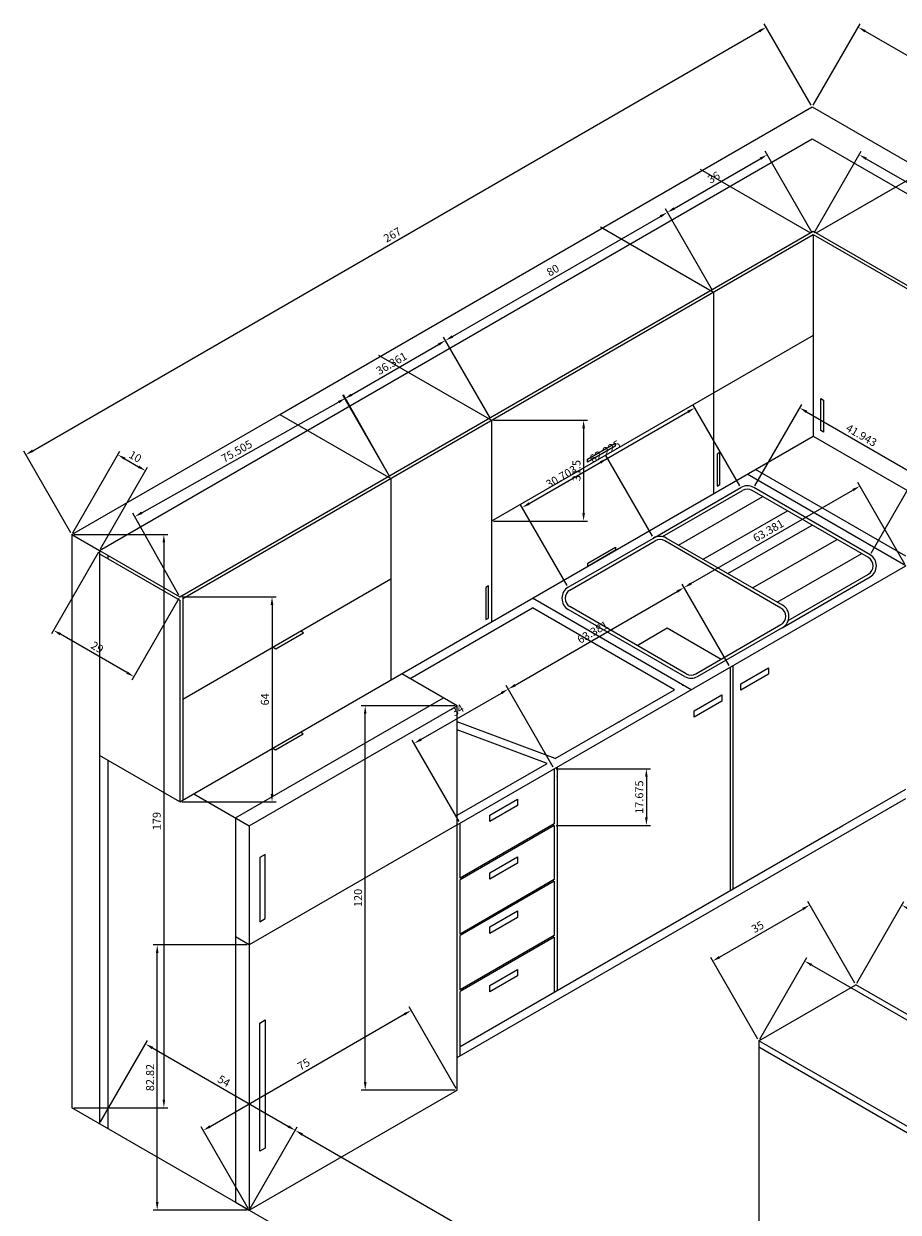
# Model space of a CAD drawing. Units: centimetres. Extents: x 239489 to 240034, y 95136 to 95693.
# Tile 2 of 4: x 239489 to 239762, y 95322 to 95693. Entities that reach past the tile are written whole.
import ezdxf

# ---------------------------------------------------------------- set-up
doc = ezdxf.new("R2010")
doc.units = ezdxf.units.CM
doc.layers.add('A-ANNO-DIMS', color=2, linetype='Continuous', lineweight=18)
doc.layers.add('A-FLOR-CASE', color=7, linetype='Continuous', lineweight=25)
doc.styles.get("Standard").update_dxf_attribs({"font": 'arial.ttf'})
doc.dimstyles.new('ISO-25', dxfattribs={"dimtxt": 2.5, "dimasz": 2.5, "dimexe": 1.25, "dimexo": 0.625, "dimtad": 1, "dimdec": 1, "dimdsep": 46, "dimtxsty": 'Standard', "dimcen": 2.5, "dimadec": 0, "dimazin": 0, "dimtfac": 1, "dimtdec": 1, "dimtmove": 0, "dimatfit": 3, "dimfxl": 1, "dimarcsym": 0})

# ---------------------------------------------------------------- blocks, each defined once
blk = doc.blocks.new('HANDLE-DOOR')
for p, q in [((0.87, 10.5), (0, 10)), ((0, 10), (0, 0)), ((0.87, 0.5), (0.87, 10.5)), ((0, 0), (0.87, 0.5))]:
    blk.add_line(p, q)
blk = doc.blocks.new('HANDLE-DRAWER')
for p, q in [((0, 2), (8.66, 7)), ((8.66, 5), (0, 0)), ((8.66, 7), (8.66, 5)), ((0, 0), (0, 2))]:
    blk.add_line(p, q)
blk = doc.blocks.new('*D4')
at = {"layer": 'A-ANNO-DIMS', "color": 0, "lineweight": -2, "transparency": 16777216}
for p, q in [((239734.94, 95667.89), (239720.25, 95693.33)), ((239491.82, 95560), (239718.71, 95691)), ((239503.71, 95534.39), (239489.03, 95559.83))]:
    blk.add_line(p, q, dxfattribs=at)
at = {"layer": 'A-ANNO-DIMS', "color": 0, "transparency": 16777216}
for points in [[(239718.51, 95691.36), (239718.92, 95690.64), (239720.88, 95692.25)], [(239491.61, 95560.36), (239492.02, 95559.64), (239489.65, 95558.75)]]:
    blk.add_solid(points, dxfattribs=at)
at = {"layer": 'Defpoints', "color": 0, "transparency": 16777216}
for p in [(239720.88, 95692.25), (239735.25, 95667.35), (239504.03, 95533.85)]:
    blk.add_point(p, dxfattribs=at)
at = {"layer": 'A-ANNO-DIMS', "color": 0, "transparency": 16777216, "insert": (239604.31, 95627.15), "char_height": 2.5, "attachment_point": 5, "rotation": 30}
blk.add_mtext('267', dxfattribs=at)
blk = doc.blocks.new('*D5')
at = {"layer": 'A-ANNO-DIMS', "color": 0, "lineweight": -2, "transparency": 16777216}
for p, q in [((239735.57, 95667.89), (239750.25, 95693.33)), ((239751.79, 95691), (239980.86, 95558.75)), ((239968.97, 95533.14), (239983.65, 95558.58))]:
    blk.add_line(p, q, dxfattribs=at)
at = {"layer": 'A-ANNO-DIMS', "color": 0, "transparency": 16777216}
for points in [[(239752, 95691.36), (239751.59, 95690.64), (239749.63, 95692.25)], [(239981.07, 95559.11), (239980.65, 95558.39), (239983.03, 95557.5)]]:
    blk.add_solid(points, dxfattribs=at)
at = {"layer": 'Defpoints', "color": 0, "transparency": 16777216}
for p in [(239735.25, 95667.35), (239983.03, 95557.5), (239968.65, 95532.6)]:
    blk.add_point(p, dxfattribs=at)
at = {"layer": 'A-ANNO-DIMS', "color": 0, "transparency": 16777216, "insert": (239867.28, 95626.52), "char_height": 2.5, "attachment_point": 5, "rotation": 330}
blk.add_mtext('269.505', dxfattribs=at)
blk = doc.blocks.new('*D7')
at = {"layer": 'A-ANNO-DIMS', "color": 0, "lineweight": -2, "transparency": 16777216}
for p, q in [((239504.65, 95533.85), (239534.03, 95533.85)), ((239532.78, 95531.35), (239532.78, 95357.35)), ((239504.65, 95354.85), (239534.03, 95354.85))]:
    blk.add_line(p, q, dxfattribs=at)
at = {"layer": 'A-ANNO-DIMS', "color": 0, "transparency": 16777216}
for points in [[(239532.36, 95531.35), (239533.19, 95531.35), (239532.78, 95533.85)], [(239532.36, 95357.35), (239533.19, 95357.35), (239532.78, 95354.85)]]:
    blk.add_solid(points, dxfattribs=at)
at = {"layer": 'Defpoints', "color": 0, "transparency": 16777216}
for p in [(239504.03, 95533.85), (239504.03, 95354.85), (239532.78, 95354.85)]:
    blk.add_point(p, dxfattribs=at)
at = {"layer": 'A-ANNO-DIMS', "color": 0, "transparency": 16777216, "insert": (239530.87, 95444.35), "char_height": 2.5, "attachment_point": 5, "rotation": 90}
blk.add_mtext('179', dxfattribs=at)
blk = doc.blocks.new('*D8')
at = {"layer": 'A-ANNO-DIMS', "color": 0, "lineweight": -2, "transparency": 16777216}
for p, q in [((239504.34, 95534.39), (239519.03, 95559.83)), ((239513, 95529.39), (239527.69, 95554.83)), ((239520.57, 95557.5), (239524.9, 95555))]:
    blk.add_line(p, q, dxfattribs=at)
at = {"layer": 'A-ANNO-DIMS', "color": 0, "transparency": 16777216}
for points in [[(239520.77, 95557.86), (239520.36, 95557.14), (239518.4, 95558.75)], [(239525.1, 95555.36), (239524.69, 95554.64), (239527.06, 95553.75)]]:
    blk.add_solid(points, dxfattribs=at)
at = {"layer": 'Defpoints', "color": 0, "transparency": 16777216}
for p in [(239527.06, 95553.75), (239504.03, 95533.85), (239512.69, 95528.85)]:
    blk.add_point(p, dxfattribs=at)
at = {"layer": 'A-ANNO-DIMS', "color": 0, "transparency": 16777216, "insert": (239523.68, 95557.9), "char_height": 2.5, "attachment_point": 5, "rotation": 330}
blk.add_mtext('10', dxfattribs=at)
blk = doc.blocks.new('*D10')
at = {"layer": 'A-ANNO-DIMS', "color": 0, "lineweight": -2, "transparency": 16777216}
for p, q in [((239513, 95350.39), (239527.69, 95375.83)), ((239529.23, 95373.5), (239571.66, 95349)), ((239559.76, 95323.39), (239574.45, 95348.83))]:
    blk.add_line(p, q, dxfattribs=at)
at = {"layer": 'A-ANNO-DIMS', "color": 0, "transparency": 16777216}
for points in [[(239529.43, 95373.86), (239529.02, 95373.14), (239527.06, 95374.75)], [(239571.87, 95349.36), (239571.45, 95348.64), (239573.83, 95347.75)]]:
    blk.add_solid(points, dxfattribs=at)
at = {"layer": 'Defpoints', "color": 0, "transparency": 16777216}
for p in [(239512.69, 95349.85), (239573.83, 95347.75), (239559.45, 95322.85)]:
    blk.add_point(p, dxfattribs=at)
at = {"layer": 'A-ANNO-DIMS', "color": 0, "transparency": 16777216, "insert": (239551.39, 95362.89), "char_height": 2.5, "attachment_point": 5, "rotation": 330}
blk.add_mtext('54', dxfattribs=at)
blk = doc.blocks.new('*D11')
at = {"layer": 'A-ANNO-DIMS', "color": 0, "lineweight": -2, "transparency": 16777216}
for p, q in [((239559.76, 95323.39), (239574.45, 95348.83)), ((239575.99, 95346.5), (239730.75, 95257.15)), ((239718.86, 95231.54), (239733.54, 95256.98))]:
    blk.add_line(p, q, dxfattribs=at)
at = {"layer": 'A-ANNO-DIMS', "color": 0, "transparency": 16777216}
for points in [[(239576.2, 95346.86), (239575.78, 95346.14), (239573.83, 95347.75)], [(239730.96, 95257.51), (239730.55, 95256.79), (239732.92, 95255.9)]]:
    blk.add_solid(points, dxfattribs=at)
at = {"layer": 'Defpoints', "color": 0, "transparency": 16777216}
for p in [(239559.45, 95322.85), (239732.92, 95255.9), (239718.54, 95231)]:
    blk.add_point(p, dxfattribs=at)
at = {"layer": 'A-ANNO-DIMS', "color": 0, "transparency": 16777216, "insert": (239654.32, 95303.47), "char_height": 2.5, "attachment_point": 5, "rotation": 330}
blk.add_mtext('183.705', dxfattribs=at)
blk = doc.blocks.new('*D12')
at = {"layer": 'A-ANNO-DIMS', "color": 0, "lineweight": -2, "transparency": 16777216}
for p, q in [((239624.09, 95360.89), (239609.4, 95386.33)), ((239547.24, 95349), (239607.86, 95384)), ((239559.14, 95323.39), (239544.45, 95348.83))]:
    blk.add_line(p, q, dxfattribs=at)
at = {"layer": 'A-ANNO-DIMS', "color": 0, "transparency": 16777216}
for points in [[(239607.66, 95384.36), (239608.07, 95383.64), (239610.03, 95385.25)], [(239547.03, 95349.36), (239547.45, 95348.64), (239545.08, 95347.75)]]:
    blk.add_solid(points, dxfattribs=at)
at = {"layer": 'Defpoints', "color": 0, "transparency": 16777216}
for p in [(239610.03, 95385.25), (239624.4, 95360.35), (239559.45, 95322.85)]:
    blk.add_point(p, dxfattribs=at)
at = {"layer": 'A-ANNO-DIMS', "color": 0, "transparency": 16777216, "insert": (239576.6, 95368.14), "char_height": 2.5, "attachment_point": 5, "rotation": 30}
blk.add_mtext('75', dxfattribs=at)
blk = doc.blocks.new('*D13')
at = {"layer": 'A-ANNO-DIMS', "color": 0, "lineweight": -2, "transparency": 16777216}
for p, q in [((239623.78, 95480.35), (239594.4, 95480.35)), ((239595.65, 95362.85), (239595.65, 95477.85)), ((239623.78, 95360.35), (239594.4, 95360.35))]:
    blk.add_line(p, q, dxfattribs=at)
at = {"layer": 'A-ANNO-DIMS', "color": 0, "transparency": 16777216}
for points in [[(239595.24, 95477.85), (239596.07, 95477.85), (239595.65, 95480.35)], [(239595.24, 95362.85), (239596.07, 95362.85), (239595.65, 95360.35)]]:
    blk.add_solid(points, dxfattribs=at)
at = {"layer": 'Defpoints', "color": 0, "transparency": 16777216}
for p in [(239595.65, 95480.35), (239624.4, 95480.35), (239624.4, 95360.35)]:
    blk.add_point(p, dxfattribs=at)
at = {"layer": 'A-ANNO-DIMS', "color": 0, "transparency": 16777216, "insert": (239593.75, 95420.35), "char_height": 2.5, "attachment_point": 5, "rotation": 90}
blk.add_mtext('120', dxfattribs=at)
blk = doc.blocks.new('*D14')
at = {"layer": 'A-ANNO-DIMS', "color": 0, "lineweight": -2, "transparency": 16777216}
for p, q in [((239558.83, 95405.67), (239529.45, 95405.67)), ((239530.7, 95325.35), (239530.7, 95403.17)), ((239558.83, 95322.85), (239529.45, 95322.85))]:
    blk.add_line(p, q, dxfattribs=at)
at = {"layer": 'A-ANNO-DIMS', "color": 0, "transparency": 16777216}
for points in [[(239530.28, 95403.17), (239531.12, 95403.17), (239530.7, 95405.67)], [(239530.28, 95325.35), (239531.12, 95325.35), (239530.7, 95322.85)]]:
    blk.add_solid(points, dxfattribs=at)
at = {"layer": 'Defpoints', "color": 0, "transparency": 16777216}
for p in [(239530.7, 95405.67), (239559.45, 95405.67), (239559.45, 95322.85)]:
    blk.add_point(p, dxfattribs=at)
at = {"layer": 'A-ANNO-DIMS', "color": 0, "transparency": 16777216, "insert": (239528.8, 95364.26), "char_height": 2.5, "attachment_point": 5, "rotation": 90}
blk.add_mtext('82.82', dxfattribs=at)
blk = doc.blocks.new('*D15')
at = {"layer": 'A-ANNO-DIMS', "color": 0, "lineweight": -2, "transparency": 16777216}
for p, q in [((239538.43, 95514.35), (239567.8, 95514.35)), ((239566.55, 95511.85), (239566.55, 95452.85)), ((239538.43, 95450.35), (239567.8, 95450.35))]:
    blk.add_line(p, q, dxfattribs=at)
at = {"layer": 'A-ANNO-DIMS', "color": 0, "transparency": 16777216}
for points in [[(239566.13, 95511.85), (239566.97, 95511.85), (239566.55, 95514.35)], [(239566.13, 95452.85), (239566.97, 95452.85), (239566.55, 95450.35)]]:
    blk.add_solid(points, dxfattribs=at)
at = {"layer": 'Defpoints', "color": 0, "transparency": 16777216}
for p in [(239537.8, 95514.35), (239537.8, 95450.35), (239566.55, 95450.35)]:
    blk.add_point(p, dxfattribs=at)
at = {"layer": 'A-ANNO-DIMS', "color": 0, "transparency": 16777216, "insert": (239564.65, 95482.35), "char_height": 2.5, "attachment_point": 5, "rotation": 90}
blk.add_mtext('64', dxfattribs=at)
blk = doc.blocks.new('*D16')
at = {"layer": 'A-ANNO-DIMS', "color": 0, "lineweight": -2, "transparency": 16777216}
for p, q in [((239512.37, 95528.31), (239497.69, 95502.87)), ((239537.49, 95513.81), (239522.8, 95488.37)), ((239521.26, 95490.7), (239500.48, 95502.7))]:
    blk.add_line(p, q, dxfattribs=at)
at = {"layer": 'A-ANNO-DIMS', "color": 0, "transparency": 16777216}
for points in [[(239500.68, 95503.06), (239500.27, 95502.34), (239498.31, 95503.95)], [(239521.47, 95491.06), (239521.05, 95490.34), (239523.43, 95489.45)]]:
    blk.add_solid(points, dxfattribs=at)
at = {"layer": 'Defpoints', "color": 0, "transparency": 16777216}
for p in [(239512.69, 95528.85), (239537.8, 95514.35), (239498.31, 95503.95)]:
    blk.add_point(p, dxfattribs=at)
at = {"layer": 'A-ANNO-DIMS', "color": 0, "transparency": 16777216, "insert": (239511.82, 95498.35), "char_height": 2.5, "attachment_point": 5, "rotation": 330}
blk.add_mtext('29', dxfattribs=at)
blk = doc.blocks.new('*D17')
at = {"layer": 'A-ANNO-DIMS', "color": 0, "lineweight": -2, "transparency": 16777216}
for p, q in [((239603.31, 95551.89), (239588.92, 95577.5)), ((239525.89, 95540.64), (239587.35, 95575.19)), ((239537.49, 95514.89), (239523.1, 95540.5))]:
    blk.add_line(p, q, dxfattribs=at)
at = {"layer": 'A-ANNO-DIMS', "color": 0, "transparency": 16777216}
for points in [[(239587.15, 95575.55), (239587.56, 95574.82), (239589.53, 95576.41)], [(239525.69, 95541), (239526.1, 95540.27), (239523.71, 95539.41)]]:
    blk.add_solid(points, dxfattribs=at)
at = {"layer": 'Defpoints', "color": 0, "transparency": 16777216}
for p in [(239589.53, 95576.41), (239603.62, 95551.35), (239537.8, 95514.35)]:
    blk.add_point(p, dxfattribs=at)
at = {"layer": 'A-ANNO-DIMS', "color": 0, "transparency": 16777216, "insert": (239555.69, 95559.57), "char_height": 2.5, "attachment_point": 5, "rotation": 29.3428}
blk.add_mtext('75.505', dxfattribs=at)
blk = doc.blocks.new('*D18')
at = {"layer": 'A-ANNO-DIMS', "color": 0, "lineweight": -2, "transparency": 16777216}
for p, q in [((239591.41, 95577.5), (239618.57, 95593.18)), ((239634.8, 95570.07), (239620.11, 95595.51)), ((239603.31, 95551.89), (239588.62, 95577.33))]:
    blk.add_line(p, q, dxfattribs=at)
at = {"layer": 'A-ANNO-DIMS', "color": 0, "transparency": 16777216}
for points in [[(239618.36, 95593.54), (239618.78, 95592.82), (239620.73, 95594.43)], [(239591.2, 95577.86), (239591.62, 95577.14), (239589.24, 95576.25)]]:
    blk.add_solid(points, dxfattribs=at)
at = {"layer": 'Defpoints', "color": 0, "transparency": 16777216}
for p in [(239620.73, 95594.43), (239635.11, 95569.53), (239603.62, 95551.35)]:
    blk.add_point(p, dxfattribs=at)
at = {"layer": 'A-ANNO-DIMS', "color": 0, "transparency": 16777216, "insert": (239604.04, 95586.99), "char_height": 2.5, "attachment_point": 5, "rotation": 30}
blk.add_mtext('36.361', dxfattribs=at)
blk = doc.blocks.new('*D19')
at = {"layer": 'A-ANNO-DIMS', "color": 0, "lineweight": -2, "transparency": 16777216}
for p, q in [((239622.9, 95595.68), (239687.85, 95633.18)), ((239704.08, 95610.07), (239689.39, 95635.51)), ((239634.8, 95570.07), (239620.11, 95595.51))]:
    blk.add_line(p, q, dxfattribs=at)
at = {"layer": 'A-ANNO-DIMS', "color": 0, "transparency": 16777216}
for points in [[(239687.64, 95633.54), (239688.06, 95632.82), (239690.02, 95634.43)], [(239622.69, 95596.04), (239623.11, 95595.32), (239620.73, 95594.43)]]:
    blk.add_solid(points, dxfattribs=at)
at = {"layer": 'Defpoints', "color": 0, "transparency": 16777216}
for p in [(239690.02, 95634.43), (239704.39, 95609.53), (239635.11, 95569.53)]:
    blk.add_point(p, dxfattribs=at)
at = {"layer": 'A-ANNO-DIMS', "color": 0, "transparency": 16777216, "insert": (239654.42, 95616.08), "char_height": 2.5, "attachment_point": 5, "rotation": 30}
blk.add_mtext('80', dxfattribs=at)
blk = doc.blocks.new('*D20')
at = {"layer": 'A-ANNO-DIMS', "color": 0, "lineweight": -2, "transparency": 16777216}
for p, q in [((239735.25, 95628.07), (239720.57, 95653.51)), ((239692.18, 95635.68), (239719.03, 95651.18)), ((239704.08, 95610.07), (239689.39, 95635.51))]:
    blk.add_line(p, q, dxfattribs=at)
at = {"layer": 'A-ANNO-DIMS', "color": 0, "transparency": 16777216}
for points in [[(239718.82, 95651.54), (239719.24, 95650.82), (239721.19, 95652.43)], [(239691.97, 95636.04), (239692.39, 95635.32), (239690.02, 95634.43)]]:
    blk.add_solid(points, dxfattribs=at)
at = {"layer": 'Defpoints', "color": 0, "transparency": 16777216}
for p in [(239721.19, 95652.43), (239735.57, 95627.53), (239704.39, 95609.53)]:
    blk.add_point(p, dxfattribs=at)
at = {"layer": 'A-ANNO-DIMS', "color": 0, "transparency": 16777216, "insert": (239704.65, 95645.08), "char_height": 2.5, "attachment_point": 5, "rotation": 30}
blk.add_mtext('36', dxfattribs=at)
blk = doc.blocks.new('*D21')
at = {"layer": 'A-ANNO-DIMS', "color": 0, "lineweight": -2, "transparency": 16777216}
for p, q in [((239635.73, 95569.53), (239665.11, 95569.53)), ((239663.86, 95567.03), (239663.86, 95540.53)), ((239635.73, 95538.03), (239665.11, 95538.03))]:
    blk.add_line(p, q, dxfattribs=at)
at = {"layer": 'A-ANNO-DIMS', "color": 0, "transparency": 16777216}
for points in [[(239663.44, 95567.03), (239664.28, 95567.03), (239663.86, 95569.53)], [(239663.44, 95540.53), (239664.28, 95540.53), (239663.86, 95538.03)]]:
    blk.add_solid(points, dxfattribs=at)
at = {"layer": 'Defpoints', "color": 0, "transparency": 16777216}
for p in [(239635.11, 95569.53), (239635.11, 95538.03), (239663.86, 95538.03)]:
    blk.add_point(p, dxfattribs=at)
at = {"layer": 'A-ANNO-DIMS', "color": 0, "transparency": 16777216, "insert": (239661.96, 95553.78), "char_height": 2.5, "attachment_point": 5, "rotation": 90}
blk.add_mtext('31.5', dxfattribs=at)
blk = doc.blocks.new('*D22')
at = {"layer": 'A-ANNO-DIMS', "color": 0, "lineweight": -2, "transparency": 16777216}
for p, q in [((239735.88, 95628.07), (239750.57, 95653.51)), ((239752.11, 95651.18), (239793.24, 95627.43)), ((239781.35, 95601.82), (239796.03, 95627.26))]:
    blk.add_line(p, q, dxfattribs=at)
at = {"layer": 'A-ANNO-DIMS', "color": 0, "transparency": 16777216}
for points in [[(239752.32, 95651.54), (239751.9, 95650.82), (239749.94, 95652.43)], [(239793.45, 95627.79), (239793.04, 95627.07), (239795.41, 95626.18)]]:
    blk.add_solid(points, dxfattribs=at)
at = {"layer": 'Defpoints', "color": 0, "transparency": 16777216}
for p in [(239735.57, 95627.53), (239795.41, 95626.18), (239781.03, 95601.28)]:
    blk.add_point(p, dxfattribs=at)
at = {"layer": 'A-ANNO-DIMS', "color": 0, "transparency": 16777216, "insert": (239773.63, 95640.95), "char_height": 2.5, "attachment_point": 5, "rotation": 330}
blk.add_mtext('52.5', dxfattribs=at)
blk = doc.blocks.new('*D30')
at = {"layer": 'A-ANNO-DIMS', "color": 0, "lineweight": -2, "transparency": 16777216}
for p, q in [((239613.06, 95469.82), (239638.17, 95484.32)), ((239654.4, 95461.21), (239639.71, 95486.65)), ((239624.96, 95444.21), (239610.27, 95469.65))]:
    blk.add_line(p, q, dxfattribs=at)
at = {"layer": 'A-ANNO-DIMS', "color": 0, "transparency": 16777216}
for points in [[(239637.97, 95484.68), (239638.38, 95483.96), (239640.34, 95485.57)], [(239612.85, 95470.18), (239613.27, 95469.46), (239610.89, 95468.57)]]:
    blk.add_solid(points, dxfattribs=at)
at = {"layer": 'Defpoints', "color": 0, "transparency": 16777216}
for p in [(239640.34, 95485.57), (239654.71, 95460.67), (239625.27, 95443.67)]:
    blk.add_point(p, dxfattribs=at)
at = {"layer": 'A-ANNO-DIMS', "color": 0, "transparency": 16777216, "insert": (239624.67, 95478.72), "char_height": 2.5, "attachment_point": 5, "rotation": 30}
blk.add_mtext('34', dxfattribs=at)
blk = doc.blocks.new('*D31')
at = {"layer": 'A-ANNO-DIMS', "color": 0, "lineweight": -2, "transparency": 16777216}
for p, q in [((239709.29, 95492.9), (239694.6, 95518.34)), ((239642.5, 95486.82), (239693.06, 95516.01)), ((239654.4, 95461.21), (239639.71, 95486.65))]:
    blk.add_line(p, q, dxfattribs=at)
at = {"layer": 'A-ANNO-DIMS', "color": 0, "transparency": 16777216}
for points in [[(239692.86, 95516.37), (239693.27, 95515.65), (239695.23, 95517.26)], [(239642.3, 95487.18), (239642.71, 95486.46), (239640.34, 95485.57)]]:
    blk.add_solid(points, dxfattribs=at)
at = {"layer": 'Defpoints', "color": 0, "transparency": 16777216}
for p in [(239695.23, 95517.26), (239709.6, 95492.36), (239654.71, 95460.67)]:
    blk.add_point(p, dxfattribs=at)
at = {"layer": 'A-ANNO-DIMS', "color": 0, "transparency": 16777216, "insert": (239666.83, 95503.06), "char_height": 2.5, "attachment_point": 5, "rotation": 30}
blk.add_mtext('63.381', dxfattribs=at)
blk = doc.blocks.new('*D32')
at = {"layer": 'A-ANNO-DIMS', "color": 0, "lineweight": -2, "transparency": 16777216}
for p, q in [((239697.39, 95518.51), (239747.95, 95547.7)), ((239764.18, 95524.59), (239749.49, 95550.03)), ((239709.29, 95492.9), (239694.6, 95518.34))]:
    blk.add_line(p, q, dxfattribs=at)
at = {"layer": 'A-ANNO-DIMS', "color": 0, "transparency": 16777216}
for points in [[(239747.75, 95548.06), (239748.16, 95547.34), (239750.12, 95548.95)], [(239697.19, 95518.87), (239697.6, 95518.15), (239695.23, 95517.26)]]:
    blk.add_solid(points, dxfattribs=at)
at = {"layer": 'Defpoints', "color": 0, "transparency": 16777216}
for p in [(239750.12, 95548.95), (239764.49, 95524.05), (239709.6, 95492.36)]:
    blk.add_point(p, dxfattribs=at)
at = {"layer": 'A-ANNO-DIMS', "color": 0, "transparency": 16777216, "insert": (239721.72, 95534.75), "char_height": 2.5, "attachment_point": 5, "rotation": 30}
blk.add_mtext('63.381', dxfattribs=at)
blk = doc.blocks.new('*D37')
at = {"layer": 'A-ANNO-DIMS', "color": 0, "lineweight": -2, "transparency": 16777216}
for p, q in [((239655.34, 95460.67), (239684.71, 95460.67)), ((239683.46, 95458.17), (239683.46, 95445.5)), ((239655.34, 95443), (239684.71, 95443))]:
    blk.add_line(p, q, dxfattribs=at)
at = {"layer": 'A-ANNO-DIMS', "color": 0, "transparency": 16777216}
for points in [[(239683.05, 95458.17), (239683.88, 95458.17), (239683.46, 95460.67)], [(239683.05, 95445.5), (239683.88, 95445.5), (239683.46, 95443)]]:
    blk.add_solid(points, dxfattribs=at)
at = {"layer": 'Defpoints', "color": 0, "transparency": 16777216}
for p in [(239654.71, 95460.67), (239654.71, 95443), (239683.46, 95443)]:
    blk.add_point(p, dxfattribs=at)
at = {"layer": 'A-ANNO-DIMS', "color": 0, "transparency": 16777216, "insert": (239681.56, 95451.83), "char_height": 2.5, "attachment_point": 5, "rotation": 90}
blk.add_mtext('17.675', dxfattribs=at)
blk = doc.blocks.new('*D38')
at = {"layer": 'A-ANNO-DIMS', "color": 0, "lineweight": -2, "transparency": 16777216}
for p, q in [((239712.66, 95549.03), (239697.97, 95574.47)), ((239646.88, 95543.52), (239696.43, 95572.13)), ((239658.77, 95517.92), (239644.09, 95543.35))]:
    blk.add_line(p, q, dxfattribs=at)
at = {"layer": 'A-ANNO-DIMS', "color": 0, "transparency": 16777216}
for points in [[(239696.23, 95572.5), (239696.64, 95571.77), (239698.6, 95573.38)], [(239646.67, 95543.88), (239647.08, 95543.16), (239644.71, 95542.27)]]:
    blk.add_solid(points, dxfattribs=at)
at = {"layer": 'Defpoints', "color": 0, "transparency": 16777216}
for p in [(239698.6, 95573.38), (239712.97, 95548.49), (239659.09, 95517.37)]:
    blk.add_point(p, dxfattribs=at)
at = {"layer": 'A-ANNO-DIMS', "color": 0, "transparency": 16777216, "insert": (239670.7, 95559.48), "char_height": 2.5, "attachment_point": 5, "rotation": 30}
blk.add_mtext('62.225', dxfattribs=at)
blk = doc.blocks.new('*D39')
at = {"layer": 'A-ANNO-DIMS', "color": 0, "lineweight": -2, "transparency": 16777216}
for p, q in [((239717.29, 95549.03), (239731.97, 95574.47)), ((239733.51, 95572.13), (239765.51, 95553.66)), ((239753.61, 95528.06), (239768.3, 95553.5))]:
    blk.add_line(p, q, dxfattribs=at)
at = {"layer": 'A-ANNO-DIMS', "color": 0, "transparency": 16777216}
for points in [[(239733.72, 95572.5), (239733.31, 95571.77), (239731.35, 95573.38)], [(239765.72, 95554.02), (239765.3, 95553.3), (239767.67, 95552.41)]]:
    blk.add_solid(points, dxfattribs=at)
at = {"layer": 'Defpoints', "color": 0, "transparency": 16777216}
for p in [(239767.67, 95552.41), (239716.97, 95548.49), (239753.3, 95527.52)]:
    blk.add_point(p, dxfattribs=at)
at = {"layer": 'A-ANNO-DIMS', "color": 0, "transparency": 16777216, "insert": (239750.46, 95564.55), "char_height": 2.5, "attachment_point": 5, "rotation": 330}
blk.add_mtext('41.943', dxfattribs=at)
blk = doc.blocks.new('*D44')
at = {"layer": 'A-ANNO-DIMS', "color": 0, "lineweight": -2, "transparency": 16777216}
for p, q in [((239718.86, 95376.27), (239733.54, 95401.71)), ((239735.08, 95399.38), (239812.26, 95354.82)), ((239800.36, 95329.21), (239815.05, 95354.65))]:
    blk.add_line(p, q, dxfattribs=at)
at = {"layer": 'A-ANNO-DIMS', "color": 0, "transparency": 16777216}
for points in [[(239735.29, 95399.74), (239734.88, 95399.02), (239732.92, 95400.63)], [(239812.47, 95355.18), (239812.05, 95354.46), (239814.42, 95353.57)]]:
    blk.add_solid(points, dxfattribs=at)
at = {"layer": 'Defpoints', "color": 0, "transparency": 16777216}
for p in [(239718.54, 95375.73), (239814.42, 95353.57), (239800.05, 95328.67)]:
    blk.add_point(p, dxfattribs=at)
at = {"layer": 'A-ANNO-DIMS', "color": 0, "transparency": 16777216, "insert": (239774.62, 95378.75), "char_height": 2.5, "attachment_point": 5, "rotation": 330}
blk.add_mtext('94.114', dxfattribs=at)
blk = doc.blocks.new('*D45')
at = {"layer": 'A-ANNO-DIMS', "color": 0, "lineweight": -2, "transparency": 16777216}
for p, q in [((239748.54, 95393.77), (239733.86, 95419.21)), ((239706.33, 95401.88), (239732.32, 95416.88)), ((239718.23, 95376.27), (239703.54, 95401.71))]:
    blk.add_line(p, q, dxfattribs=at)
at = {"layer": 'A-ANNO-DIMS', "color": 0, "transparency": 16777216}
for points in [[(239732.11, 95417.24), (239732.52, 95416.52), (239734.48, 95418.13)], [(239706.13, 95402.24), (239706.54, 95401.52), (239704.17, 95400.63)]]:
    blk.add_solid(points, dxfattribs=at)
at = {"layer": 'Defpoints', "color": 0, "transparency": 16777216}
for p in [(239734.48, 95418.13), (239748.86, 95393.23), (239718.54, 95375.73)]:
    blk.add_point(p, dxfattribs=at)
at = {"layer": 'A-ANNO-DIMS', "color": 0, "transparency": 16777216, "insert": (239718.37, 95411.02), "char_height": 2.5, "attachment_point": 5, "rotation": 30}
blk.add_mtext('35', dxfattribs=at)
blk = doc.blocks.new('*D46')
at = {"layer": 'A-ANNO-DIMS', "color": 0, "lineweight": -2, "transparency": 16777216}
for p, q in [((239749.17, 95393.77), (239763.86, 95419.21)), ((239765.4, 95416.88), (239812.38, 95389.75)), ((239800.48, 95364.15), (239815.17, 95389.59))]:
    blk.add_line(p, q, dxfattribs=at)
at = {"layer": 'A-ANNO-DIMS', "color": 0, "transparency": 16777216}
for points in [[(239765.6, 95417.24), (239765.19, 95416.52), (239763.23, 95418.13)], [(239812.58, 95390.11), (239812.17, 95389.39), (239814.54, 95388.5)]]:
    blk.add_solid(points, dxfattribs=at)
at = {"layer": 'Defpoints', "color": 0, "transparency": 16777216}
for p in [(239748.86, 95393.23), (239814.54, 95388.5), (239800.17, 95363.61)]:
    blk.add_point(p, dxfattribs=at)
at = {"layer": 'A-ANNO-DIMS', "color": 0, "transparency": 16777216, "insert": (239789.84, 95404.96), "char_height": 2.5, "attachment_point": 5, "rotation": 330}
blk.add_mtext('59.247', dxfattribs=at)
blk = doc.blocks.new('*D48')
at = {"layer": 'A-ANNO-DIMS', "color": 0, "lineweight": -2, "transparency": 16777216}
for p, q in [((239685.36, 95533.27), (239670.68, 95558.71)), ((239646.88, 95543.52), (239669.14, 95556.37)), ((239658.77, 95517.92), (239644.09, 95543.35))]:
    blk.add_line(p, q, dxfattribs=at)
at = {"layer": 'A-ANNO-DIMS', "color": 0, "transparency": 16777216}
for points in [[(239668.93, 95556.73), (239669.34, 95556.01), (239671.3, 95557.62)], [(239646.67, 95543.88), (239647.08, 95543.16), (239644.71, 95542.27)]]:
    blk.add_solid(points, dxfattribs=at)
at = {"layer": 'Defpoints', "color": 0, "transparency": 16777216}
for p in [(239671.3, 95557.62), (239685.68, 95532.73), (239659.09, 95517.37)]:
    blk.add_point(p, dxfattribs=at)
at = {"layer": 'A-ANNO-DIMS', "color": 0, "transparency": 16777216, "insert": (239657.05, 95551.6), "char_height": 2.5, "attachment_point": 5, "rotation": 30}
blk.add_mtext('30.703', dxfattribs=at)

msp = doc.modelspace()

# ---------------------------------------------------------------- linework, layer by layer
at = {"layer": 'A-ANNO-DIMS'}
for p in [(239694.8113, 95486.8198), (239674.9737, 95475.3666), (239655.5805, 95458.3607)]:
    msp.add_point(p, dxfattribs=at)
at = {"layer": 'A-FLOR-CASE'}
for p, q in [((239669.4369, 95629.3502), (239735.2548, 95667.3502)), ((239735.2548, 95667.3502), (239968.6531, 95532.5976)), ((239512.6863, 95528.8502), (239735.2548, 95657.3502)), ((239735.2548, 95657.3502), (239947.431, 95534.8502)), ((239700.3013, 95647.8914), (239734.7013, 95628.0306)), ((239669.4369, 95629.3502), (239700.6138, 95647.3502)), ((239736.4333, 95628.0306), (239769.8958, 95647.3502)), ((239736.4333, 95628.0306), (239761.2356, 95642.3502)), ((239600.1548, 95589.3502), (239669.4369, 95629.3502)), ((239669.1244, 95629.8914), (239669.7494, 95629.5306)), ((239669.1244, 95629.8914), (239704.3904, 95609.5306)), ((239537.801, 95514.3502), (239735.5673, 95628.5306)), ((239538.667, 95513.8502), (239735.5673, 95627.5306)), ((239735.5673, 95628.5306), (239921.7628, 95521.0306)), ((239735.5673, 95627.5306), (239735.5673, 95564.5306)), ((239735.5673, 95627.5306), (239921.7628, 95520.0306)), ((239704.3904, 95609.5306), (239704.3904, 95546.5306)), ((239735.5673, 95596.0306), (239635.1084, 95538.0306)), ((239568.9779, 95571.3502), (239600.1548, 95589.3502)), ((239599.8423, 95589.8914), (239635.1084, 95569.5306)), ((239504.026, 95533.8502), (239568.9779, 95571.3502)), ((239568.9779, 95571.3502), (239603.6189, 95551.3502)), ((239635.1084, 95569.5306), (239635.1084, 95506.5306)), ((239537.801, 95450.3502), (239735.5673, 95564.5306)), ((239735.5673, 95564.5306), (239780.6006, 95538.5306)), ((239603.6189, 95551.3502), (239603.6189, 95488.3502)), ((239764.4941, 95524.0512), (239714.9746, 95552.6414)), ((239764.4941, 95527.0512), (239717.5726, 95554.1414)), ((239685.5193, 95532.6354), (239712.9746, 95548.4867)), ((239688.4665, 95533.1822), (239713.4746, 95547.6206)), ((239752.798, 95526.6493), (239716.4746, 95547.6206)), ((239753.298, 95527.5153), (239716.9746, 95548.4867)), ((239693.4475, 95530.5474), (239719.8512, 95545.6711)), ((239701.1604, 95526.0944), (239727.5642, 95541.218)), ((239708.8734, 95521.6413), (239735.2771, 95536.765)), ((239504.026, 95533.8502), (239512.6863, 95528.8502)), ((239504.026, 95533.8502), (239504.026, 95354.8502)), ((239659.086, 95517.3741), (239685.6752, 95532.7254)), ((239725.9986, 95511.754), (239689.6752, 95532.7254)), ((239512.6863, 95528.8502), (239537.801, 95514.3502)), ((239512.6863, 95528.8502), (239512.6863, 95349.8502)), ((239659.586, 95516.508), (239686.1752, 95531.8593)), ((239725.4986, 95510.888), (239689.1752, 95531.8593)), ((239716.5863, 95517.1882), (239742.99, 95532.3119)), ((239512.6863, 95527.8502), (239537.801, 95513.3502)), ((239515.2844, 95527.3502), (239515.2844, 95526.3502)), ((239724.2992, 95512.7352), (239750.703, 95527.8588)), ((239624.4036, 95443.1699), (239764.4941, 95524.0512)), ((239727.7899, 95507.0147), (239752.798, 95521.4531)), ((239603.6189, 95519.8502), (239538.667, 95482.3502)), ((239725.8427, 95504.7358), (239753.298, 95520.5871)), ((239537.801, 95513.3502), (239537.801, 95450.3502)), ((239538.667, 95513.8502), (239538.667, 95450.8502)), ((239609.6811, 95488.8502), (239647.8898, 95510.91)), ((239697.4094, 95485.3198), (239647.8898, 95513.91)), ((239692.2132, 95485.3198), (239647.8898, 95510.91)), ((239695.4094, 95489.4745), (239659.086, 95510.4459)), ((239695.9094, 95490.3405), (239659.586, 95511.3119)), ((239567.7373, 95498.1339), (239576.3976, 95503.1339)), ((239576.3976, 95503.1339), (239575.5315, 95503.6339)), ((239680.554, 95499.206), (239689.9963, 95504.6574)), ((239689.9963, 95504.6574), (239706.8516, 95494.926)), ((239698.9094, 95490.3405), (239725.4986, 95505.6919)), ((239699.4094, 95489.4745), (239725.9986, 95504.8258)), ((239566.8713, 95498.6339), (239567.7373, 95498.1339)), ((239709.6043, 95492.3606), (239709.6043, 95422.6613)), ((239710.4703, 95492.8606), (239710.4703, 95423.1613)), ((239624.4036, 95480.3502), (239607.083, 95490.3502)), ((239655.0259, 95463.8497), (239692.2132, 95485.3198)), ((239655.0259, 95463.8497), (239692.2132, 95485.3198)), ((239555.1215, 95445.3502), (239620.0734, 95482.8502)), ((239559.4517, 95442.8502), (239624.4036, 95480.3502)), ((239624.4036, 95360.3502), (239624.4036, 95480.3502)), ((239655.0259, 95463.8497), (239624.4036, 95475.3096)), ((239567.6551, 95466.5864), (239576.3154, 95471.5864)), ((239576.3154, 95471.5864), (239575.4493, 95472.0864)), ((239652.4278, 95462.3497), (239624.4036, 95472.8373)), ((239566.7891, 95467.0864), (239567.6551, 95466.5864)), ((239537.801, 95450.3502), (239512.6863, 95464.8502)), ((239515.2844, 95463.3502), (239515.2844, 95348.3502)), ((239624.4036, 95446.1699), (239652.4278, 95462.3497)), ((239654.7144, 95460.6699), (239654.7144, 95443.5307)), ((239655.5805, 95461.1699), (239655.5805, 95391.4707)), ((239542.1311, 95452.8502), (239559.4517, 95442.8502)), ((239624.4036, 95370.4707), (239764.4941, 95451.352)), ((239744.7811, 95442.9707), (239764.4941, 95454.352)), ((239555.1215, 95445.3502), (239555.1215, 95325.3502)), ((239625.2696, 95426.5307), (239625.2696, 95443.6699)), ((239654.7144, 95443.5307), (239625.2696, 95426.5307)), ((239624.4036, 95443.1699), (239559.4517, 95405.6699)), ((239559.4517, 95442.8502), (239559.4517, 95322.8502)), ((239654.7144, 95442.9951), (239625.2696, 95425.9951)), ((239625.2696, 95373.9707), (239744.7811, 95442.9707)), ((239654.7144, 95442.9951), (239654.7144, 95426.0703)), ((239564.443, 95433.9249), (239562.711, 95432.9249)), ((239562.711, 95432.9249), (239562.711, 95412.9249)), ((239564.443, 95413.9249), (239564.443, 95433.9249)), ((239654.7144, 95426.0703), (239625.2696, 95409.0703)), ((239625.2696, 95409.0703), (239625.2696, 95425.9951)), ((239654.7144, 95425.5703), (239625.2696, 95408.5703)), ((239654.7144, 95425.5703), (239654.7144, 95408.6455)), ((239562.711, 95412.9249), (239564.443, 95413.9249)), ((239559.4517, 95405.6699), (239555.1215, 95408.1699)), ((239654.7144, 95408.6455), (239625.2696, 95391.6455)), ((239625.2696, 95391.6455), (239625.2696, 95408.5703)), ((239654.7144, 95408.1455), (239625.2696, 95391.1455)), ((239654.7144, 95408.1455), (239654.7144, 95390.9707)), ((239718.5446, 95375.7293), (239748.8555, 95393.2293)), ((239800.1652, 95363.6056), (239748.8555, 95393.2293)), ((239625.2696, 95370.9707), (239625.2696, 95391.1455)), ((239562.711, 95381.2458), (239564.443, 95382.2458)), ((239562.711, 95341.2458), (239562.711, 95381.2458)), ((239564.443, 95382.2458), (239564.443, 95342.2458)), ((239800.0497, 95328.6722), (239718.5446, 95375.7293)), ((239718.5446, 95375.7293), (239718.5446, 95230.9978)), ((239800.0497, 95326.6722), (239718.5446, 95373.7293)), ((239559.4517, 95322.8502), (239624.4036, 95360.3502)), ((239559.4517, 95322.8502), (239504.026, 95354.8502)), ((239564.443, 95342.2458), (239562.711, 95341.2458)), ((239555.1215, 95325.3502), (239559.4517, 95322.8502)), ((239559.4517, 95322.8502), (239800.0497, 95183.9408))]:
    msp.add_line(p, q, dxfattribs=at)
for centre, radius, start, end in [((239714.9746, 95545.0226), 4, 60, 120), ((239714.9746, 95545.0226), 3, 60, 120), ((239687.6752, 95529.2613), 4, 60, 120), ((239687.6752, 95529.2613), 3, 60, 120), ((239751.298, 95524.0512), 3, 300, 60), ((239751.298, 95524.0512), 4, 300, 60), ((239661.086, 95513.91), 4, 120, 240), ((239661.086, 95513.91), 3, 120, 240), ((239723.9986, 95508.2899), 3, 300, 60), ((239723.9986, 95508.2899), 4, 300, 60), ((239697.4094, 95492.9386), 4, 240, 300), ((239697.4094, 95492.9386), 3, 240, 300)]:
    msp.add_arc(centre, radius, start, end, dxfattribs=at)

# ---------------------------------------------------------------- block references
at = {"layer": 'A-FLOR-CASE', "extrusion": (0, 0, -1), "zscale": -1}
for p, rotation in [((-239737.9135, 95576.3354), 180), ((-239673.7577, 95562.4068), 240.0000000006339), ((-239673.8563, 95529.9012), 240.0000000004035)]:
    msp.add_blockref('HANDLE-DOOR', p, dxfattribs=dict(at, rotation=rotation))
at = {"layer": 'A-FLOR-CASE', "rotation": 180}
msp.add_blockref('HANDLE-DOOR', (239706.4035, 95559.4707), dxfattribs=at)
at = {"layer": 'A-FLOR-CASE'}
for name, p in [('HANDLE-DOOR', (239633.298, 95507.263)), ('HANDLE-DRAWER', (239712.9143, 95485.1876)), ('HANDLE-DRAWER', (239698.3363, 95476.771)), ('HANDLE-DRAWER', (239634.53, 95444.176)), ('HANDLE-DRAWER', (239634.53, 95426.2275)), ('HANDLE-DRAWER', (239634.53, 95409.2867)), ('HANDLE-DRAWER', (239634.53, 95391.0028))]:
    msp.add_blockref(name, p, dxfattribs=at)

# ---------------------------------------------------------------- dimensions: what is measured, and where the dimension line sits
at = {"layer": 'A-ANNO-DIMS'}
for base, p1, p2, angle, override, picture, middle in [((239720.8798, 95692.2484), (239504.026, 95533.8502), (239735.2548, 95667.3502), 30, {"dimdec": 0, "dimlfac": 1, "dimrnd": 0, "dimzin": 0, "dimdsep": 46, "dimlunit": 2}, '*D4', (239604.3147, 95627.1451)), ((239983.0281, 95557.4959), (239735.2548, 95667.3502), (239968.6531, 95532.5976), 330, {"dimdec": 3, "dimlfac": 1, "dimrnd": 0, "dimzin": 0, "dimdsep": 46, "dimlunit": 2}, '*D5', (239867.2796, 95626.5188)), ((239721.1923, 95652.4288), (239704.3904, 95609.5306), (239735.5673, 95627.5306), 30, {"dimdec": 0, "dimlfac": 1, "dimrnd": 0, "dimzin": 0, "dimdsep": 46, "dimlunit": 2}, '*D20', (239704.6527, 95645.0762)), ((239795.4086, 95626.1788), (239735.5673, 95627.5306), (239781.0336, 95601.2806), 330, {"dimdec": 1, "dimlfac": 1, "dimrnd": 0, "dimzin": 0, "dimdsep": 46, "dimlunit": 2}, '*D22', (239773.6262, 95640.9505)), ((239690.0154, 95634.4288), (239635.1084, 95569.5306), (239704.3904, 95609.5306), 30, {"dimdec": 0, "dimlfac": 1, "dimrnd": 0, "dimzin": 0, "dimdsep": 46, "dimlunit": 2}, '*D19', (239654.4237, 95616.0755)), ((239620.7334, 95594.4288), (239603.6189, 95551.3502), (239635.1084, 95569.5306), 30, {"dimdec": 3, "dimlfac": 1, "dimrnd": 0, "dimzin": 0, "dimdsep": 46, "dimlunit": 2}, '*D18', (239604.0375, 95586.986)), ((239589.5305, 95576.4116), (239537.801, 95514.3502), (239603.6189, 95551.3502), 29.342816, {"dimdec": 3, "dimlfac": 1, "dimrnd": 0, "dimzin": 0, "dimdsep": 46, "dimlunit": 2}, '*D17', (239555.6897, 95559.5691)), ((239698.5996, 95573.3849), (239659.086, 95517.3741), (239712.9746, 95548.4867), 30, {"dimdec": 3, "dimlfac": 1, "dimrnd": 0, "dimzin": 0, "dimdsep": 46, "dimlunit": 2}, '*D38', (239670.7045, 95559.4753)), ((239767.673, 95552.4136), (239716.9746, 95548.4867), (239753.298, 95527.5153), 330, {"dimdec": 3, "dimlfac": 1, "dimrnd": 0, "dimzin": 0, "dimdsep": 46, "dimlunit": 2}, '*D39', (239750.4624, 95564.5466)), ((239663.8584, 95538.0306), (239635.1084, 95569.5306), (239635.1084, 95538.0306), 270, {"dimdec": 1, "dimlfac": 1, "dimrnd": 0, "dimzin": 0, "dimdsep": 46, "dimlunit": 2}, '*D21', (239661.9561, 95553.7806)), ((239527.0613, 95553.7484), (239504.026, 95533.8502), (239512.6863, 95528.8502), 330, {"dimdec": 0, "dimlfac": 1, "dimrnd": 0, "dimzin": 0, "dimdsep": 46, "dimlunit": 2}, '*D8', (239523.6819, 95557.8951)), ((239671.3002, 95557.6236), (239659.086, 95517.3741), (239685.6752, 95532.7254), 30, {"dimdec": 3, "dimlfac": 1, "dimrnd": 0, "dimzin": 0, "dimdsep": 46, "dimlunit": 2}, '*D48', (239657.0544, 95551.5954)), ((239750.1191, 95548.9495), (239709.6043, 95492.3606), (239764.4941, 95524.0512), 30, {"dimdec": 3, "dimlfac": 1, "dimrnd": 0, "dimzin": 0, "dimdsep": 46, "dimlunit": 2}, '*D32', (239721.7231, 95534.7515)), ((239532.776, 95354.8502), (239504.026, 95533.8502), (239504.026, 95354.8502), 270, {"dimdec": 0, "dimlfac": 1, "dimrnd": 0, "dimzin": 0, "dimdsep": 46, "dimlunit": 2}, '*D7', (239530.8746, 95444.3502)), ((239498.3113, 95503.9519), (239537.801, 95514.3502), (239512.6863, 95528.8502), 150, {"dimdec": 0, "dimlfac": 1, "dimrnd": 0, "dimzin": 0, "dimdsep": 46, "dimlunit": 2}, '*D16', (239511.8194, 95498.3486)), ((239695.2293, 95517.2588), (239654.7144, 95460.6699), (239709.6043, 95492.3606), 30, {"dimdec": 3, "dimlfac": 1, "dimrnd": 0, "dimzin": 0, "dimdsep": 46, "dimlunit": 2}, '*D31', (239666.8332, 95503.0609)), ((239566.551, 95450.3502), (239537.801, 95514.3502), (239537.801, 95450.3502), 270, {"dimdec": 0, "dimlfac": 1, "dimrnd": 0, "dimzin": 0, "dimdsep": 46, "dimlunit": 2}, '*D15', (239564.6496, 95482.3502)), ((239640.3394, 95485.5681), (239625.2696, 95443.6699), (239654.7144, 95460.6699), 30, {"dimdec": 0, "dimlfac": 1, "dimrnd": 0, "dimzin": 0, "dimdsep": 46, "dimlunit": 2}, '*D30', (239624.6659, 95478.7156)), ((239595.6536, 95480.3502), (239624.4036, 95360.3502), (239624.4036, 95480.3502), 90, {"dimdec": 0, "dimlfac": 1, "dimrnd": 0, "dimzin": 0, "dimdsep": 46, "dimlunit": 2}, '*D13', (239593.7521, 95420.3502)), ((239683.4644, 95442.9951), (239654.7144, 95460.6699), (239654.7144, 95442.9951), 270, {"dimdec": 3, "dimlfac": 1, "dimrnd": 0, "dimzin": 0, "dimdsep": 46, "dimlunit": 2}, '*D37', (239681.563, 95451.8325)), ((239734.4805, 95418.1275), (239718.5446, 95375.7293), (239748.8555, 95393.2293), 30, {"dimdec": 0, "dimlfac": 1, "dimrnd": 0, "dimzin": 0, "dimdsep": 46, "dimlunit": 2}, '*D45', (239718.3739, 95411.0249)), ((239814.5402, 95388.5038), (239748.8555, 95393.2293), (239800.1652, 95363.6056), 330, {"dimdec": 3, "dimlfac": 1, "dimrnd": 0, "dimzin": 0, "dimdsep": 46, "dimlunit": 2}, '*D46', (239789.836, 95404.9623)), ((239530.7017, 95405.6699), (239559.4517, 95322.8502), (239559.4517, 95405.6699), 90, {"dimdec": 2, "dimlfac": 1, "dimrnd": 0, "dimzin": 0, "dimdsep": 46, "dimlunit": 2}, '*D14', (239528.8002, 95364.26)), ((239814.4247, 95353.5704), (239718.5446, 95375.7293), (239800.0497, 95328.6722), 330, {"dimdec": 3, "dimlfac": 1, "dimrnd": 0, "dimzin": 0, "dimdsep": 46, "dimlunit": 2}, '*D44', (239774.6229, 95378.7457)), ((239610.0286, 95385.2484), (239559.4517, 95322.8502), (239624.4036, 95360.3502), 30, {"dimdec": 0, "dimlfac": 1, "dimrnd": 0, "dimzin": 0, "dimdsep": 46, "dimlunit": 2}, '*D12', (239576.6044, 95368.1407)), ((239573.8267, 95347.7484), (239512.6863, 95349.8502), (239559.4517, 95322.8502), 330, {"dimdec": 0, "dimlfac": 1, "dimrnd": 0, "dimzin": 0, "dimdsep": 46, "dimlunit": 2}, '*D10', (239551.3921, 95362.8907)), ((239732.9196, 95255.8961), (239559.4517, 95322.8502), (239718.5446, 95230.9978), 330, {"dimdec": 3, "dimlfac": 1, "dimrnd": 0, "dimzin": 0, "dimdsep": 46, "dimlunit": 2}, '*D11', (239654.3243, 95303.4697))]:
    dim = msp.add_linear_dim(base=base, p1=p1, p2=p2, angle=angle, dimstyle='ISO-25', override=override, dxfattribs=at)
    dim.commit()
    dim.dimension.update_dxf_attribs({"geometry": picture, "text_midpoint": middle})

doc.saveas('drawing.dxf')
